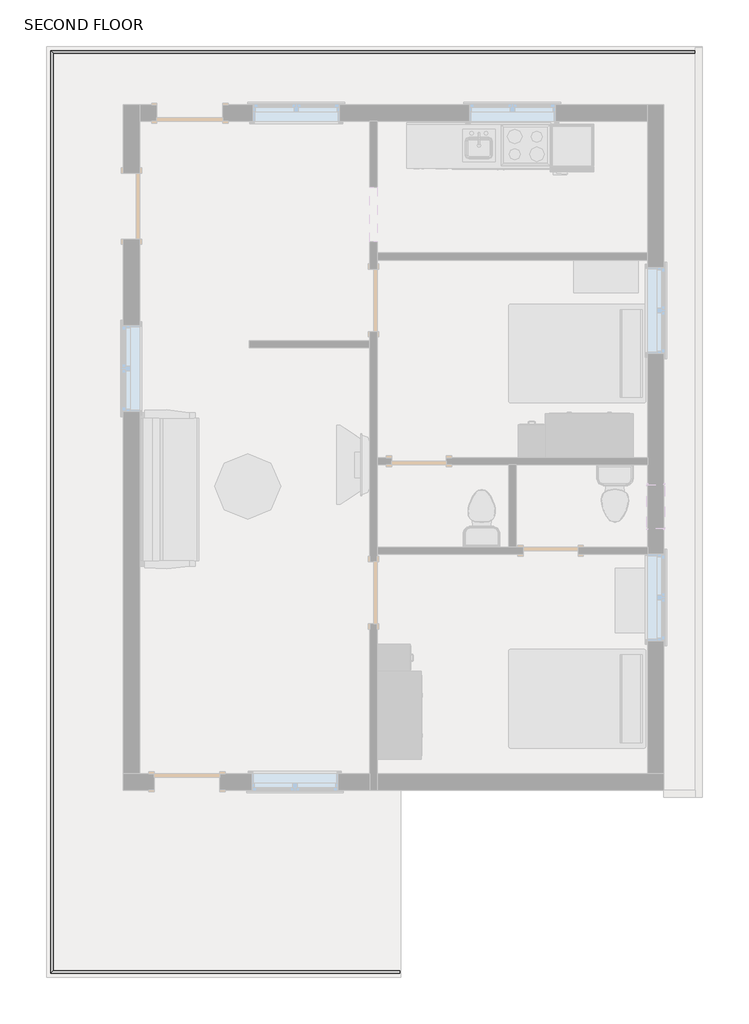
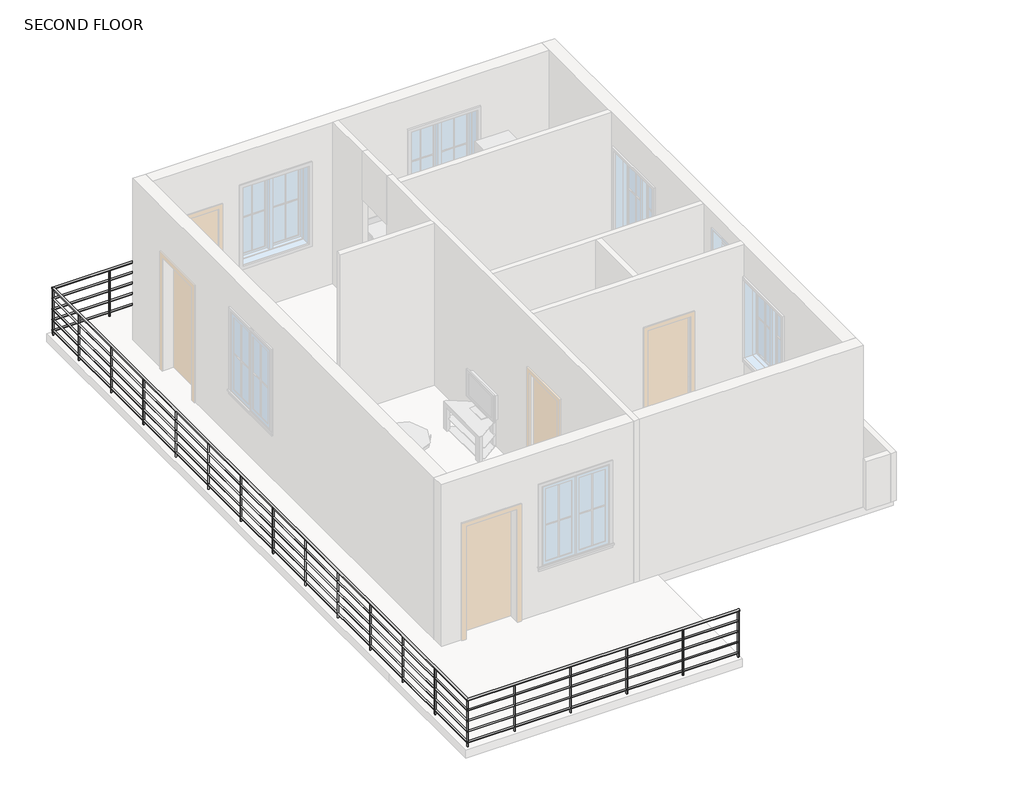
# One storey, part 2 of 3: 1 railing.
"""IFC4 building model written with IfcOpenShell, lengths in millimetres."""

from ifc_helpers import new_model, si_unit, point, frame, frame_2d, origin, place, context, project, spatial, circle_curve, ellipse_curve, trimmed, segment, composite_curve, outline, extrude, element, save
from ifc_brep_helpers import plane_surface, cylinder_surface, advanced_brep

model = new_model("IFC4")

# Units and contexts
model_context = context("Model", 3, world=origin())
ifc_project = project(units=[si_unit("LENGTHUNIT", "METRE", prefix="MILLI")], contexts=[model_context])

# Site, building, storey
site = spatial("IfcSite", under=ifc_project)
building = spatial("IfcBuilding", under=site)
storey = spatial("IfcBuildingStorey", under=building, Name="SECOND FLOOR", Elevation=6400.8)

# Railing
placement = place(None, origin())
element("IfcRailing", 1, ObjectType="900mm Pipe", at=placement, inside=storey, context=model_context, shape_type="SolidModel", body=[
    advanced_brep(
    [(200.9145071, -6925.6741001, 7280.8), (200.9145071, -6965.6741001, 7280.8), (-4655.4544048, -6965.6741001, 7280.8), (-4615.4544048, -6925.6741001, 7280.8), (-4655.4544048, 5865.7351347, 7280.8), (-4615.4544048, 5825.7351347, 7280.8), (4406.9455952, 5825.7351347, 7280.8), (4406.9455952, 5865.7351347, 7280.8)],
    [
        (0, 1, circle_curve(frame((200.9145071, -6945.6741001, 7280.8), z_axis=(1.0, 0.0, 0.0), x_axis=(0.0, -1.0, 0.0)), 20.0)),
        (1, 0, circle_curve(frame((200.9145071, -6945.6741001, 7280.8), z_axis=(1.0, 0.0, 0.0), x_axis=(0.0, -1.0, 0.0)), 20.0)),
        (1, 2),
        (2, 3, ellipse_curve(frame((-4635.4544048, -6945.6741001, 7280.8), z_axis=(0.7071067811865458, -0.7071067811865492, 0.0), x_axis=(0.7071067811865492, 0.7071067811865458, 0.0)), 28.2842712, 20.0)),
        (3, 0),
        (3, 2, ellipse_curve(frame((-4635.4544048, -6945.6741001, 7280.8), z_axis=(0.7071067811865458, -0.7071067811865492, 0.0), x_axis=(0.7071067811865492, 0.7071067811865458, 0.0)), 28.2842712, 20.0)),
        (2, 4),
        (4, 5, ellipse_curve(frame((-4635.4544048, 5845.7351347, 7280.8), z_axis=(-0.7071067811865491, -0.7071067811865459, 0.0), x_axis=(0.7071067811865458, -0.7071067811865491, 0.0)), 28.2842712, 20.0)),
        (5, 3),
        (5, 4, ellipse_curve(frame((-4635.4544048, 5845.7351347, 7280.8), z_axis=(-0.7071067811865491, -0.7071067811865459, 0.0), x_axis=(0.7071067811865458, -0.7071067811865491, 0.0)), 28.2842712, 20.0)),
        (6, 7, circle_curve(frame((4406.9455952, 5845.7351347, 7280.8), z_axis=(1.0, 0.0, 0.0), x_axis=(0.0, 1.0, 0.0)), 20.0)),
        (7, 6, circle_curve(frame((4406.9455952, 5845.7351347, 7280.8), z_axis=(1.0, 0.0, 0.0), x_axis=(0.0, 1.0, 0.0)), 20.0)),
        (4, 7),
        (6, 5),
    ],
    [
        plane_surface(frame((200.9145071, -6945.6741001, 7300.8), z_axis=(1.0, 0.0, 0.0), x_axis=(0.0, -1.0, 0.0))),
        cylinder_surface(frame((200.9145071, -6945.6741001, 7280.8), z_axis=(1.0, 0.0, 0.0), x_axis=(0.0, -1.0, 0.0)), 20.0),
        cylinder_surface(frame((-4635.4544048, -6945.6741001, 7280.8), z_axis=(0.0, -1.0, 0.0), x_axis=(-1.0, 0.0, 0.0)), 20.0),
        plane_surface(frame((4406.9455952, 5845.7351347, 7300.8), z_axis=(1.0, 0.0, 0.0), x_axis=(0.0, 1.0, 0.0))),
        cylinder_surface(frame((-4635.4544048, 5845.7351347, 7280.8), z_axis=(-1.0, 0.0, 0.0), x_axis=(0.0, 1.0, 0.0)), 20.0),
    ],
    [
        (0, [[1, 2]]),
        (1, [[-2, 3, 4, 5]]),
        (1, [[-1, -5, 6, -3]]),
        (2, [[-4, 7, 8, 9]]),
        (2, [[-6, -9, 10, -7]]),
        (3, [[11, 12]]),
        (4, [[-8, 13, -11, 14]]),
        (4, [[-10, -14, -12, -13]]),
    ],
),
    advanced_brep(
    [(200.9145071, -6960.6741001, 7085.8), (200.9145071, -6930.6741001, 7085.8), (4406.9455952, 5860.7351347, 7085.8), (4406.9455952, 5830.7351347, 7085.8), (-4650.4544048, -6960.6741001, 7085.8), (-4620.4544048, -6930.6741001, 7085.8), (-4650.4544048, 5860.7351347, 7085.8), (-4620.4544048, 5830.7351347, 7085.8)],
    [
        (0, 1, circle_curve(frame((200.9145071, -6945.6741001, 7085.8), z_axis=(1.0, 0.0, 0.0), x_axis=(0.0, 1.0, 0.0)), 15.0)),
        (1, 0, circle_curve(frame((200.9145071, -6945.6741001, 7085.8), z_axis=(1.0, 0.0, 0.0), x_axis=(0.0, 1.0, 0.0)), 15.0)),
        (2, 3, circle_curve(frame((4406.9455952, 5845.7351347, 7085.8), z_axis=(1.0, 0.0, 0.0), x_axis=(0.0, -1.0, 0.0)), 15.0)),
        (3, 2, circle_curve(frame((4406.9455952, 5845.7351347, 7085.8), z_axis=(1.0, 0.0, 0.0), x_axis=(0.0, -1.0, 0.0)), 15.0)),
        (0, 4),
        (4, 5, ellipse_curve(frame((-4635.4544048, -6945.6741001, 7085.8), z_axis=(0.7071067811865458, -0.7071067811865492, 0.0), x_axis=(0.7071067811865492, 0.7071067811865458, 0.0)), 21.2132034, 15.0)),
        (5, 1),
        (5, 4, ellipse_curve(frame((-4635.4544048, -6945.6741001, 7085.8), z_axis=(0.7071067811865458, -0.7071067811865492, 0.0), x_axis=(0.7071067811865492, 0.7071067811865458, 0.0)), 21.2132034, 15.0)),
        (4, 6),
        (6, 7, ellipse_curve(frame((-4635.4544048, 5845.7351347, 7085.8), z_axis=(-0.7071067811865491, -0.7071067811865459, 0.0), x_axis=(0.7071067811865458, -0.7071067811865491, 0.0)), 21.2132034, 15.0)),
        (7, 5),
        (7, 6, ellipse_curve(frame((-4635.4544048, 5845.7351347, 7085.8), z_axis=(-0.7071067811865491, -0.7071067811865459, 0.0), x_axis=(0.7071067811865458, -0.7071067811865491, 0.0)), 21.2132034, 15.0)),
        (6, 2),
        (3, 7),
    ],
    [
        plane_surface(frame((200.9145071, -6945.6741001, 7100.8), z_axis=(1.0, 0.0, 0.0), x_axis=(0.0, -1.0, 0.0))),
        plane_surface(frame((4406.9455952, 5845.7351347, 7100.8), z_axis=(1.0, 0.0, 0.0), x_axis=(0.0, 1.0, 0.0))),
        cylinder_surface(frame((200.9145071, -6945.6741001, 7085.8), z_axis=(1.0, 0.0, 0.0), x_axis=(0.0, 1.0, 0.0)), 15.0),
        cylinder_surface(frame((-4635.4544048, -6945.6741001, 7085.8), z_axis=(0.0, -1.0, 0.0), x_axis=(1.0, 0.0, 0.0)), 15.0),
        cylinder_surface(frame((-4635.4544048, 5845.7351347, 7085.8), z_axis=(-1.0, 0.0, 0.0), x_axis=(0.0, -1.0, 0.0)), 15.0),
    ],
    [
        (0, [[1, 2]]),
        (1, [[3, 4]]),
        (2, [[-1, 5, 6, 7]]),
        (2, [[-2, -7, 8, -5]]),
        (3, [[-6, 9, 10, 11]]),
        (3, [[-8, -11, 12, -9]]),
        (4, [[-10, 13, -4, 14]]),
        (4, [[-12, -14, -3, -13]]),
    ],
),
    advanced_brep(
    [(200.9145071, -6960.6741001, 6885.8), (200.9145071, -6930.6741001, 6885.8), (4406.9455952, 5860.7351347, 6885.8), (4406.9455952, 5830.7351347, 6885.8), (-4650.4544048, -6960.6741001, 6885.8), (-4620.4544048, -6930.6741001, 6885.8), (-4650.4544048, 5860.7351347, 6885.8), (-4620.4544048, 5830.7351347, 6885.8)],
    [
        (0, 1, circle_curve(frame((200.9145071, -6945.6741001, 6885.8), z_axis=(1.0, 0.0, 0.0), x_axis=(0.0, 1.0, 0.0)), 15.0)),
        (1, 0, circle_curve(frame((200.9145071, -6945.6741001, 6885.8), z_axis=(1.0, 0.0, 0.0), x_axis=(0.0, 1.0, 0.0)), 15.0)),
        (2, 3, circle_curve(frame((4406.9455952, 5845.7351347, 6885.8), z_axis=(1.0, 0.0, 0.0), x_axis=(0.0, -1.0, 0.0)), 15.0)),
        (3, 2, circle_curve(frame((4406.9455952, 5845.7351347, 6885.8), z_axis=(1.0, 0.0, 0.0), x_axis=(0.0, -1.0, 0.0)), 15.0)),
        (0, 4),
        (4, 5, ellipse_curve(frame((-4635.4544048, -6945.6741001, 6885.8), z_axis=(0.7071067811865458, -0.7071067811865492, 0.0), x_axis=(0.7071067811865492, 0.7071067811865458, 0.0)), 21.2132034, 15.0)),
        (5, 1),
        (5, 4, ellipse_curve(frame((-4635.4544048, -6945.6741001, 6885.8), z_axis=(0.7071067811865458, -0.7071067811865492, 0.0), x_axis=(0.7071067811865492, 0.7071067811865458, 0.0)), 21.2132034, 15.0)),
        (4, 6),
        (6, 7, ellipse_curve(frame((-4635.4544048, 5845.7351347, 6885.8), z_axis=(-0.7071067811865491, -0.7071067811865459, 0.0), x_axis=(0.7071067811865458, -0.7071067811865491, 0.0)), 21.2132034, 15.0)),
        (7, 5),
        (7, 6, ellipse_curve(frame((-4635.4544048, 5845.7351347, 6885.8), z_axis=(-0.7071067811865491, -0.7071067811865459, 0.0), x_axis=(0.7071067811865458, -0.7071067811865491, 0.0)), 21.2132034, 15.0)),
        (6, 2),
        (3, 7),
    ],
    [
        plane_surface(frame((200.9145071, -6945.6741001, 6900.8), z_axis=(1.0, 0.0, 0.0), x_axis=(0.0, -1.0, 0.0))),
        plane_surface(frame((4406.9455952, 5845.7351347, 6900.8), z_axis=(1.0, 0.0, 0.0), x_axis=(0.0, 1.0, 0.0))),
        cylinder_surface(frame((200.9145071, -6945.6741001, 6885.8), z_axis=(1.0, 0.0, 0.0), x_axis=(0.0, 1.0, 0.0)), 15.0),
        cylinder_surface(frame((-4635.4544048, -6945.6741001, 6885.8), z_axis=(0.0, -1.0, 0.0), x_axis=(1.0, 0.0, 0.0)), 15.0),
        cylinder_surface(frame((-4635.4544048, 5845.7351347, 6885.8), z_axis=(-1.0, 0.0, 0.0), x_axis=(0.0, -1.0, 0.0)), 15.0),
    ],
    [
        (0, [[1, 2]]),
        (1, [[3, 4]]),
        (2, [[-1, 5, 6, 7]]),
        (2, [[-2, -7, 8, -5]]),
        (3, [[-6, 9, 10, 11]]),
        (3, [[-8, -11, 12, -9]]),
        (4, [[-10, 13, -4, 14]]),
        (4, [[-12, -14, -3, -13]]),
    ],
),
    advanced_brep(
    [(200.9145071, -6960.6741001, 6685.8), (200.9145071, -6930.6741001, 6685.8), (-4650.4544048, -6960.6741001, 6685.8), (-4620.4544048, -6930.6741001, 6685.8), (-4650.4544048, 5860.7351347, 6685.8), (-4620.4544048, 5830.7351347, 6685.8), (4406.9455952, 5860.7351347, 6685.8), (4406.9455952, 5830.7351347, 6685.8)],
    [
        (0, 1, circle_curve(frame((200.9145071, -6945.6741001, 6685.8), z_axis=(1.0, 0.0, 0.0), x_axis=(0.0, 1.0, 0.0)), 15.0)),
        (1, 0, circle_curve(frame((200.9145071, -6945.6741001, 6685.8), z_axis=(1.0, 0.0, 0.0), x_axis=(0.0, 1.0, 0.0)), 15.0)),
        (0, 2),
        (2, 3, ellipse_curve(frame((-4635.4544048, -6945.6741001, 6685.8), z_axis=(0.7071067811865458, -0.7071067811865492, 0.0), x_axis=(0.7071067811865492, 0.7071067811865458, 0.0)), 21.2132034, 15.0)),
        (3, 1),
        (3, 2, ellipse_curve(frame((-4635.4544048, -6945.6741001, 6685.8), z_axis=(0.7071067811865458, -0.7071067811865492, 0.0), x_axis=(0.7071067811865492, 0.7071067811865458, 0.0)), 21.2132034, 15.0)),
        (2, 4),
        (4, 5, ellipse_curve(frame((-4635.4544048, 5845.7351347, 6685.8), z_axis=(-0.7071067811865491, -0.7071067811865459, 0.0), x_axis=(0.7071067811865458, -0.7071067811865491, 0.0)), 21.2132034, 15.0)),
        (5, 3),
        (5, 4, ellipse_curve(frame((-4635.4544048, 5845.7351347, 6685.8), z_axis=(-0.7071067811865491, -0.7071067811865459, 0.0), x_axis=(0.7071067811865458, -0.7071067811865491, 0.0)), 21.2132034, 15.0)),
        (6, 7, circle_curve(frame((4406.9455952, 5845.7351347, 6685.8), z_axis=(1.0, 0.0, 0.0), x_axis=(0.0, -1.0, 0.0)), 15.0)),
        (7, 6, circle_curve(frame((4406.9455952, 5845.7351347, 6685.8), z_axis=(1.0, 0.0, 0.0), x_axis=(0.0, -1.0, 0.0)), 15.0)),
        (4, 6),
        (7, 5),
    ],
    [
        plane_surface(frame((200.9145071, -6945.6741001, 6700.8), z_axis=(1.0, 0.0, 0.0), x_axis=(0.0, -1.0, 0.0))),
        cylinder_surface(frame((200.9145071, -6945.6741001, 6685.8), z_axis=(1.0, 0.0, 0.0), x_axis=(0.0, 1.0, 0.0)), 15.0),
        cylinder_surface(frame((-4635.4544048, -6945.6741001, 6685.8), z_axis=(0.0, -1.0, 0.0), x_axis=(1.0, 0.0, 0.0)), 15.0),
        plane_surface(frame((4406.9455952, 5845.7351347, 6700.8), z_axis=(1.0, 0.0, 0.0), x_axis=(0.0, 1.0, 0.0))),
        cylinder_surface(frame((-4635.4544048, 5845.7351347, 6685.8), z_axis=(-1.0, 0.0, 0.0), x_axis=(0.0, -1.0, 0.0)), 15.0),
    ],
    [
        (0, [[1, 2]]),
        (1, [[-1, 3, 4, 5]]),
        (1, [[-2, -5, 6, -3]]),
        (2, [[-4, 7, 8, 9]]),
        (2, [[-6, -9, 10, -7]]),
        (3, [[11, 12]]),
        (4, [[-8, 13, -12, 14]]),
        (4, [[-10, -14, -11, -13]]),
    ],
),
    advanced_brep(
    [(200.9145071, -6960.6741001, 6485.8), (200.9145071, -6930.6741001, 6485.8), (-4650.4544048, -6960.6741001, 6485.8), (-4620.4544048, -6930.6741001, 6485.8), (-4650.4544048, 5860.7351347, 6485.8), (-4620.4544048, 5830.7351347, 6485.8), (4406.9455952, 5860.7351347, 6485.8), (4406.9455952, 5830.7351347, 6485.8)],
    [
        (0, 1, circle_curve(frame((200.9145071, -6945.6741001, 6485.8), z_axis=(1.0, 0.0, 0.0), x_axis=(0.0, 1.0, 0.0)), 15.0)),
        (1, 0, circle_curve(frame((200.9145071, -6945.6741001, 6485.8), z_axis=(1.0, 0.0, 0.0), x_axis=(0.0, 1.0, 0.0)), 15.0)),
        (0, 2),
        (2, 3, ellipse_curve(frame((-4635.4544048, -6945.6741001, 6485.8), z_axis=(0.7071067811865458, -0.7071067811865492, 0.0), x_axis=(0.7071067811865492, 0.7071067811865458, 0.0)), 21.2132034, 15.0)),
        (3, 1),
        (3, 2, ellipse_curve(frame((-4635.4544048, -6945.6741001, 6485.8), z_axis=(0.7071067811865458, -0.7071067811865492, 0.0), x_axis=(0.7071067811865492, 0.7071067811865458, 0.0)), 21.2132034, 15.0)),
        (2, 4),
        (4, 5, ellipse_curve(frame((-4635.4544048, 5845.7351347, 6485.8), z_axis=(-0.7071067811865491, -0.7071067811865459, 0.0), x_axis=(0.7071067811865458, -0.7071067811865491, 0.0)), 21.2132034, 15.0)),
        (5, 3),
        (5, 4, ellipse_curve(frame((-4635.4544048, 5845.7351347, 6485.8), z_axis=(-0.7071067811865491, -0.7071067811865459, 0.0), x_axis=(0.7071067811865458, -0.7071067811865491, 0.0)), 21.2132034, 15.0)),
        (6, 7, circle_curve(frame((4406.9455952, 5845.7351347, 6485.8), z_axis=(1.0, 0.0, 0.0), x_axis=(0.0, -1.0, 0.0)), 15.0)),
        (7, 6, circle_curve(frame((4406.9455952, 5845.7351347, 6485.8), z_axis=(1.0, 0.0, 0.0), x_axis=(0.0, -1.0, 0.0)), 15.0)),
        (4, 6),
        (7, 5),
    ],
    [
        plane_surface(frame((200.9145071, -6945.6741001, 6500.8), z_axis=(1.0, 0.0, 0.0), x_axis=(0.0, -1.0, 0.0))),
        cylinder_surface(frame((200.9145071, -6945.6741001, 6485.8), z_axis=(1.0, 0.0, 0.0), x_axis=(0.0, 1.0, 0.0)), 15.0),
        cylinder_surface(frame((-4635.4544048, -6945.6741001, 6485.8), z_axis=(0.0, -1.0, 0.0), x_axis=(1.0, 0.0, 0.0)), 15.0),
        plane_surface(frame((4406.9455952, 5845.7351347, 6500.8), z_axis=(1.0, 0.0, 0.0), x_axis=(0.0, 1.0, 0.0))),
        cylinder_surface(frame((-4635.4544048, 5845.7351347, 6485.8), z_axis=(-1.0, 0.0, 0.0), x_axis=(0.0, -1.0, 0.0)), 15.0),
    ],
    [
        (0, [[1, 2]]),
        (1, [[-1, 3, 4, 5]]),
        (1, [[-2, -5, 6, -3]]),
        (2, [[-4, 7, 8, 9]]),
        (2, [[-6, -9, 10, -7]]),
        (3, [[11, 12]]),
        (4, [[-8, 13, -12, 14]]),
        (4, [[-10, -14, -11, -13]]),
    ],
),
    extrude(outline(composite_curve([segment(trimmed(circle_curve(frame_2d((4364.5455952, 5845.7351347)), 12.5), [point((4364.5455952, 5858.2351347))], [point((4364.5455952, 5833.2351347))], False, "CARTESIAN"), True, "CONTINUOUS"), segment(trimmed(circle_curve(frame_2d((4364.5455952, 5845.7351347)), 12.5), [point((4364.5455952, 5833.2351347))], [point((4364.5455952, 5858.2351347))], False, "CARTESIAN"), True, "CONTINUOUS")], self_intersect=False)), frame((0.0, 0.0, 6400.8), z_axis=(0.0, 0.0, 1.0), x_axis=(1.0, 0.0, 0.0)), (0.0, 0.0, 1.0), 860.0),
    extrude(outline(composite_curve([segment(trimmed(circle_curve(frame_2d((3364.5455952, 5845.7351347)), 12.5), [point((3364.5455952, 5858.2351347))], [point((3364.5455952, 5833.2351347))], False, "CARTESIAN"), True, "CONTINUOUS"), segment(trimmed(circle_curve(frame_2d((3364.5455952, 5845.7351347)), 12.5), [point((3364.5455952, 5833.2351347))], [point((3364.5455952, 5858.2351347))], False, "CARTESIAN"), True, "CONTINUOUS")], self_intersect=False)), frame((0.0, 0.0, 6400.8), z_axis=(0.0, 0.0, 1.0), x_axis=(1.0, 0.0, 0.0)), (0.0, 0.0, 1.0), 860.0),
    extrude(outline(composite_curve([segment(trimmed(circle_curve(frame_2d((2364.5455952, 5845.7351347)), 12.5), [point((2364.5455952, 5858.2351347))], [point((2364.5455952, 5833.2351347))], False, "CARTESIAN"), True, "CONTINUOUS"), segment(trimmed(circle_curve(frame_2d((2364.5455952, 5845.7351347)), 12.5), [point((2364.5455952, 5833.2351347))], [point((2364.5455952, 5858.2351347))], False, "CARTESIAN"), True, "CONTINUOUS")], self_intersect=False)), frame((0.0, 0.0, 6400.8), z_axis=(0.0, 0.0, 1.0), x_axis=(1.0, 0.0, 0.0)), (0.0, 0.0, 1.0), 860.0),
    extrude(outline(composite_curve([segment(trimmed(circle_curve(frame_2d((1364.5455952, 5845.7351347)), 12.5), [point((1364.5455952, 5858.2351347))], [point((1364.5455952, 5833.2351347))], False, "CARTESIAN"), True, "CONTINUOUS"), segment(trimmed(circle_curve(frame_2d((1364.5455952, 5845.7351347)), 12.5), [point((1364.5455952, 5833.2351347))], [point((1364.5455952, 5858.2351347))], False, "CARTESIAN"), True, "CONTINUOUS")], self_intersect=False)), frame((0.0, 0.0, 6400.8), z_axis=(0.0, 0.0, 1.0), x_axis=(1.0, 0.0, 0.0)), (0.0, 0.0, 1.0), 860.0),
    extrude(outline(composite_curve([segment(trimmed(circle_curve(frame_2d((364.5455952, 5845.7351347)), 12.5), [point((364.5455952, 5858.2351347))], [point((364.5455952, 5833.2351347))], False, "CARTESIAN"), True, "CONTINUOUS"), segment(trimmed(circle_curve(frame_2d((364.5455952, 5845.7351347)), 12.5), [point((364.5455952, 5833.2351347))], [point((364.5455952, 5858.2351347))], False, "CARTESIAN"), True, "CONTINUOUS")], self_intersect=False)), frame((0.0, 0.0, 6400.8), z_axis=(0.0, 0.0, 1.0), x_axis=(1.0, 0.0, 0.0)), (0.0, 0.0, 1.0), 860.0),
    extrude(outline(composite_curve([segment(trimmed(circle_curve(frame_2d((-635.4544048, 5845.7351347)), 12.5), [point((-635.4544048, 5858.2351347))], [point((-635.4544048, 5833.2351347))], False, "CARTESIAN"), True, "CONTINUOUS"), segment(trimmed(circle_curve(frame_2d((-635.4544048, 5845.7351347)), 12.5), [point((-635.4544048, 5833.2351347))], [point((-635.4544048, 5858.2351347))], False, "CARTESIAN"), True, "CONTINUOUS")], self_intersect=False)), frame((0.0, 0.0, 6400.8), z_axis=(0.0, 0.0, 1.0), x_axis=(1.0, 0.0, 0.0)), (0.0, 0.0, 1.0), 860.0),
    extrude(outline(composite_curve([segment(trimmed(circle_curve(frame_2d((-1635.4544048, 5845.7351347)), 12.5), [point((-1635.4544048, 5858.2351347))], [point((-1635.4544048, 5833.2351347))], False, "CARTESIAN"), True, "CONTINUOUS"), segment(trimmed(circle_curve(frame_2d((-1635.4544048, 5845.7351347)), 12.5), [point((-1635.4544048, 5833.2351347))], [point((-1635.4544048, 5858.2351347))], False, "CARTESIAN"), True, "CONTINUOUS")], self_intersect=False)), frame((0.0, 0.0, 6400.8), z_axis=(0.0, 0.0, 1.0), x_axis=(1.0, 0.0, 0.0)), (0.0, 0.0, 1.0), 860.0),
    extrude(outline(composite_curve([segment(trimmed(circle_curve(frame_2d((-2635.4544048, 5845.7351347)), 12.5), [point((-2635.4544048, 5858.2351347))], [point((-2635.4544048, 5833.2351347))], False, "CARTESIAN"), True, "CONTINUOUS"), segment(trimmed(circle_curve(frame_2d((-2635.4544048, 5845.7351347)), 12.5), [point((-2635.4544048, 5833.2351347))], [point((-2635.4544048, 5858.2351347))], False, "CARTESIAN"), True, "CONTINUOUS")], self_intersect=False)), frame((0.0, 0.0, 6400.8), z_axis=(0.0, 0.0, 1.0), x_axis=(1.0, 0.0, 0.0)), (0.0, 0.0, 1.0), 860.0),
    extrude(outline(composite_curve([segment(trimmed(circle_curve(frame_2d((-3635.4544048, 5845.7351347)), 12.5), [point((-3635.4544048, 5858.2351347))], [point((-3635.4544048, 5833.2351347))], False, "CARTESIAN"), True, "CONTINUOUS"), segment(trimmed(circle_curve(frame_2d((-3635.4544048, 5845.7351347)), 12.5), [point((-3635.4544048, 5833.2351347))], [point((-3635.4544048, 5858.2351347))], False, "CARTESIAN"), True, "CONTINUOUS")], self_intersect=False)), frame((0.0, 0.0, 6400.8), z_axis=(0.0, 0.0, 1.0), x_axis=(1.0, 0.0, 0.0)), (0.0, 0.0, 1.0), 860.0),
    extrude(outline(composite_curve([segment(trimmed(circle_curve(frame_2d((-4635.4544048, 5054.3258999)), 12.5), [point((-4647.9544048, 5054.3258999))], [point((-4622.9544048, 5054.3258999))], False, "CARTESIAN"), True, "CONTINUOUS"), segment(trimmed(circle_curve(frame_2d((-4635.4544048, 5054.3258999)), 12.5), [point((-4622.9544048, 5054.3258999))], [point((-4647.9544048, 5054.3258999))], False, "CARTESIAN"), True, "CONTINUOUS")], self_intersect=False)), frame((0.0, 0.0, 6400.8), z_axis=(0.0, 0.0, 1.0), x_axis=(1.0, 0.0, 0.0)), (0.0, 0.0, 1.0), 860.0),
    extrude(outline(composite_curve([segment(trimmed(circle_curve(frame_2d((-4635.4544048, 4054.3258999)), 12.5), [point((-4647.9544048, 4054.3258999))], [point((-4622.9544048, 4054.3258999))], False, "CARTESIAN"), True, "CONTINUOUS"), segment(trimmed(circle_curve(frame_2d((-4635.4544048, 4054.3258999)), 12.5), [point((-4622.9544048, 4054.3258999))], [point((-4647.9544048, 4054.3258999))], False, "CARTESIAN"), True, "CONTINUOUS")], self_intersect=False)), frame((0.0, 0.0, 6400.8), z_axis=(0.0, 0.0, 1.0), x_axis=(1.0, 0.0, 0.0)), (0.0, 0.0, 1.0), 860.0),
    extrude(outline(composite_curve([segment(trimmed(circle_curve(frame_2d((-4635.4544048, 3054.3258999)), 12.5), [point((-4647.9544048, 3054.3258999))], [point((-4622.9544048, 3054.3258999))], False, "CARTESIAN"), True, "CONTINUOUS"), segment(trimmed(circle_curve(frame_2d((-4635.4544048, 3054.3258999)), 12.5), [point((-4622.9544048, 3054.3258999))], [point((-4647.9544048, 3054.3258999))], False, "CARTESIAN"), True, "CONTINUOUS")], self_intersect=False)), frame((0.0, 0.0, 6400.8), z_axis=(0.0, 0.0, 1.0), x_axis=(1.0, 0.0, 0.0)), (0.0, 0.0, 1.0), 860.0),
    extrude(outline(composite_curve([segment(trimmed(circle_curve(frame_2d((-4635.4544048, 2054.3258999)), 12.5), [point((-4647.9544048, 2054.3258999))], [point((-4622.9544048, 2054.3258999))], False, "CARTESIAN"), True, "CONTINUOUS"), segment(trimmed(circle_curve(frame_2d((-4635.4544048, 2054.3258999)), 12.5), [point((-4622.9544048, 2054.3258999))], [point((-4647.9544048, 2054.3258999))], False, "CARTESIAN"), True, "CONTINUOUS")], self_intersect=False)), frame((0.0, 0.0, 6400.8), z_axis=(0.0, 0.0, 1.0), x_axis=(1.0, 0.0, 0.0)), (0.0, 0.0, 1.0), 860.0),
    extrude(outline(composite_curve([segment(trimmed(circle_curve(frame_2d((-4635.4544048, 1054.3258999)), 12.5), [point((-4647.9544048, 1054.3258999))], [point((-4622.9544048, 1054.3258999))], False, "CARTESIAN"), True, "CONTINUOUS"), segment(trimmed(circle_curve(frame_2d((-4635.4544048, 1054.3258999)), 12.5), [point((-4622.9544048, 1054.3258999))], [point((-4647.9544048, 1054.3258999))], False, "CARTESIAN"), True, "CONTINUOUS")], self_intersect=False)), frame((0.0, 0.0, 6400.8), z_axis=(0.0, 0.0, 1.0), x_axis=(1.0, 0.0, 0.0)), (0.0, 0.0, 1.0), 860.0),
    extrude(outline(composite_curve([segment(trimmed(circle_curve(frame_2d((-4635.4544048, 54.3258999)), 12.5), [point((-4647.9544048, 54.3258999))], [point((-4622.9544048, 54.3258999))], False, "CARTESIAN"), True, "CONTINUOUS"), segment(trimmed(circle_curve(frame_2d((-4635.4544048, 54.3258999)), 12.5), [point((-4622.9544048, 54.3258999))], [point((-4647.9544048, 54.3258999))], False, "CARTESIAN"), True, "CONTINUOUS")], self_intersect=False)), frame((0.0, 0.0, 6400.8), z_axis=(0.0, 0.0, 1.0), x_axis=(1.0, 0.0, 0.0)), (0.0, 0.0, 1.0), 860.0),
    extrude(outline(composite_curve([segment(trimmed(circle_curve(frame_2d((-4635.4544048, -945.6741001)), 12.5), [point((-4647.9544048, -945.6741001))], [point((-4622.9544048, -945.6741001))], False, "CARTESIAN"), True, "CONTINUOUS"), segment(trimmed(circle_curve(frame_2d((-4635.4544048, -945.6741001)), 12.5), [point((-4622.9544048, -945.6741001))], [point((-4647.9544048, -945.6741001))], False, "CARTESIAN"), True, "CONTINUOUS")], self_intersect=False)), frame((0.0, 0.0, 6400.8), z_axis=(0.0, 0.0, 1.0), x_axis=(1.0, 0.0, 0.0)), (0.0, 0.0, 1.0), 860.0),
    extrude(outline(composite_curve([segment(trimmed(circle_curve(frame_2d((-4635.4544048, -1945.6741001)), 12.5), [point((-4647.9544048, -1945.6741001))], [point((-4622.9544048, -1945.6741001))], False, "CARTESIAN"), True, "CONTINUOUS"), segment(trimmed(circle_curve(frame_2d((-4635.4544048, -1945.6741001)), 12.5), [point((-4622.9544048, -1945.6741001))], [point((-4647.9544048, -1945.6741001))], False, "CARTESIAN"), True, "CONTINUOUS")], self_intersect=False)), frame((0.0, 0.0, 6400.8), z_axis=(0.0, 0.0, 1.0), x_axis=(1.0, 0.0, 0.0)), (0.0, 0.0, 1.0), 860.0),
    extrude(outline(composite_curve([segment(trimmed(circle_curve(frame_2d((-4635.4544048, -2945.6741001)), 12.5), [point((-4647.9544048, -2945.6741001))], [point((-4622.9544048, -2945.6741001))], False, "CARTESIAN"), True, "CONTINUOUS"), segment(trimmed(circle_curve(frame_2d((-4635.4544048, -2945.6741001)), 12.5), [point((-4622.9544048, -2945.6741001))], [point((-4647.9544048, -2945.6741001))], False, "CARTESIAN"), True, "CONTINUOUS")], self_intersect=False)), frame((0.0, 0.0, 6400.8), z_axis=(0.0, 0.0, 1.0), x_axis=(1.0, 0.0, 0.0)), (0.0, 0.0, 1.0), 860.0),
    extrude(outline(composite_curve([segment(trimmed(circle_curve(frame_2d((-4635.4544048, -3945.6741001)), 12.5), [point((-4647.9544048, -3945.6741001))], [point((-4622.9544048, -3945.6741001))], False, "CARTESIAN"), True, "CONTINUOUS"), segment(trimmed(circle_curve(frame_2d((-4635.4544048, -3945.6741001)), 12.5), [point((-4622.9544048, -3945.6741001))], [point((-4647.9544048, -3945.6741001))], False, "CARTESIAN"), True, "CONTINUOUS")], self_intersect=False)), frame((0.0, 0.0, 6400.8), z_axis=(0.0, 0.0, 1.0), x_axis=(1.0, 0.0, 0.0)), (0.0, 0.0, 1.0), 860.0),
    extrude(outline(composite_curve([segment(trimmed(circle_curve(frame_2d((-4635.4544048, -4945.6741001)), 12.5), [point((-4647.9544048, -4945.6741001))], [point((-4622.9544048, -4945.6741001))], False, "CARTESIAN"), True, "CONTINUOUS"), segment(trimmed(circle_curve(frame_2d((-4635.4544048, -4945.6741001)), 12.5), [point((-4622.9544048, -4945.6741001))], [point((-4647.9544048, -4945.6741001))], False, "CARTESIAN"), True, "CONTINUOUS")], self_intersect=False)), frame((0.0, 0.0, 6400.8), z_axis=(0.0, 0.0, 1.0), x_axis=(1.0, 0.0, 0.0)), (0.0, 0.0, 1.0), 860.0),
    extrude(outline(composite_curve([segment(trimmed(circle_curve(frame_2d((-4635.4544048, -5945.6741001)), 12.5), [point((-4647.9544048, -5945.6741001))], [point((-4622.9544048, -5945.6741001))], False, "CARTESIAN"), True, "CONTINUOUS"), segment(trimmed(circle_curve(frame_2d((-4635.4544048, -5945.6741001)), 12.5), [point((-4622.9544048, -5945.6741001))], [point((-4647.9544048, -5945.6741001))], False, "CARTESIAN"), True, "CONTINUOUS")], self_intersect=False)), frame((0.0, 0.0, 6400.8), z_axis=(0.0, 0.0, 1.0), x_axis=(1.0, 0.0, 0.0)), (0.0, 0.0, 1.0), 860.0),
    extrude(outline(composite_curve([segment(trimmed(circle_curve(frame_2d((-3799.0854929, -6945.6741001)), 12.5), [point((-3799.0854929, -6958.1741001))], [point((-3799.0854929, -6933.1741001))], False, "CARTESIAN"), True, "CONTINUOUS"), segment(trimmed(circle_curve(frame_2d((-3799.0854929, -6945.6741001)), 12.5), [point((-3799.0854929, -6933.1741001))], [point((-3799.0854929, -6958.1741001))], False, "CARTESIAN"), True, "CONTINUOUS")], self_intersect=False)), frame((0.0, 0.0, 6400.8), z_axis=(0.0, 0.0, 1.0), x_axis=(1.0, 0.0, 0.0)), (0.0, 0.0, 1.0), 860.0),
    extrude(outline(composite_curve([segment(trimmed(circle_curve(frame_2d((-2799.0854929, -6945.6741001)), 12.5), [point((-2799.0854929, -6958.1741001))], [point((-2799.0854929, -6933.1741001))], False, "CARTESIAN"), True, "CONTINUOUS"), segment(trimmed(circle_curve(frame_2d((-2799.0854929, -6945.6741001)), 12.5), [point((-2799.0854929, -6933.1741001))], [point((-2799.0854929, -6958.1741001))], False, "CARTESIAN"), True, "CONTINUOUS")], self_intersect=False)), frame((0.0, 0.0, 6400.8), z_axis=(0.0, 0.0, 1.0), x_axis=(1.0, 0.0, 0.0)), (0.0, 0.0, 1.0), 860.0),
    extrude(outline(composite_curve([segment(trimmed(circle_curve(frame_2d((-1799.0854929, -6945.6741001)), 12.5), [point((-1799.0854929, -6958.1741001))], [point((-1799.0854929, -6933.1741001))], False, "CARTESIAN"), True, "CONTINUOUS"), segment(trimmed(circle_curve(frame_2d((-1799.0854929, -6945.6741001)), 12.5), [point((-1799.0854929, -6933.1741001))], [point((-1799.0854929, -6958.1741001))], False, "CARTESIAN"), True, "CONTINUOUS")], self_intersect=False)), frame((0.0, 0.0, 6400.8), z_axis=(0.0, 0.0, 1.0), x_axis=(1.0, 0.0, 0.0)), (0.0, 0.0, 1.0), 860.0),
    extrude(outline(composite_curve([segment(trimmed(circle_curve(frame_2d((-799.0854929, -6945.6741001)), 12.5), [point((-799.0854929, -6958.1741001))], [point((-799.0854929, -6933.1741001))], False, "CARTESIAN"), True, "CONTINUOUS"), segment(trimmed(circle_curve(frame_2d((-799.0854929, -6945.6741001)), 12.5), [point((-799.0854929, -6933.1741001))], [point((-799.0854929, -6958.1741001))], False, "CARTESIAN"), True, "CONTINUOUS")], self_intersect=False)), frame((0.0, 0.0, 6400.8), z_axis=(0.0, 0.0, 1.0), x_axis=(1.0, 0.0, 0.0)), (0.0, 0.0, 1.0), 860.0),
    extrude(outline(composite_curve([segment(trimmed(circle_curve(frame_2d((-4635.4544048, 5845.7351347)), 12.5), [point((-4647.9544048, 5845.7351347))], [point((-4622.9544048, 5845.7351347))], False, "CARTESIAN"), True, "CONTINUOUS"), segment(trimmed(circle_curve(frame_2d((-4635.4544048, 5845.7351347)), 12.5), [point((-4622.9544048, 5845.7351347))], [point((-4647.9544048, 5845.7351347))], False, "CARTESIAN"), True, "CONTINUOUS")], self_intersect=False)), frame((0.0, 0.0, 6400.8), z_axis=(0.0, 0.0, 1.0), x_axis=(1.0, 0.0, 0.0)), (0.0, 0.0, 1.0), 860.0),
    extrude(outline(composite_curve([segment(trimmed(circle_curve(frame_2d((-4635.4544048, -6945.6741001)), 12.5), [point((-4635.4544048, -6958.1741001))], [point((-4635.4544048, -6933.1741001))], False, "CARTESIAN"), True, "CONTINUOUS"), segment(trimmed(circle_curve(frame_2d((-4635.4544048, -6945.6741001)), 12.5), [point((-4635.4544048, -6933.1741001))], [point((-4635.4544048, -6958.1741001))], False, "CARTESIAN"), True, "CONTINUOUS")], self_intersect=False)), frame((0.0, 0.0, 6400.8), z_axis=(0.0, 0.0, 1.0), x_axis=(1.0, 0.0, 0.0)), (0.0, 0.0, 1.0), 860.0),
    extrude(outline(composite_curve([segment(trimmed(circle_curve(frame_2d((4394.4455952, 5845.7351347)), 12.5), [point((4394.4455952, 5858.2351347))], [point((4394.4455952, 5833.2351347))], False, "CARTESIAN"), True, "CONTINUOUS"), segment(trimmed(circle_curve(frame_2d((4394.4455952, 5845.7351347)), 12.5), [point((4394.4455952, 5833.2351347))], [point((4394.4455952, 5858.2351347))], False, "CARTESIAN"), True, "CONTINUOUS")], self_intersect=False)), frame((0.0, 0.0, 6400.8), z_axis=(0.0, 0.0, 1.0), x_axis=(1.0, 0.0, 0.0)), (0.0, 0.0, 1.0), 860.0),
    extrude(outline(composite_curve([segment(trimmed(circle_curve(frame_2d((188.4145071, -6945.6741001)), 12.5), [point((188.4145071, -6958.1741001))], [point((188.4145071, -6933.1741001))], False, "CARTESIAN"), True, "CONTINUOUS"), segment(trimmed(circle_curve(frame_2d((188.4145071, -6945.6741001)), 12.5), [point((188.4145071, -6933.1741001))], [point((188.4145071, -6958.1741001))], False, "CARTESIAN"), True, "CONTINUOUS")], self_intersect=False)), frame((0.0, 0.0, 6400.8), z_axis=(0.0, 0.0, 1.0), x_axis=(1.0, 0.0, 0.0)), (0.0, 0.0, 1.0), 860.0),
])

save(model, "model.ifc")

# Revit data of these elements
# Type "900mm Pipe"
#   built-in parameter 1008612 = 0.019685 (stored number, unit not read)
#   built-in parameter 1008611 = 0.0984252 (stored number, unit not read)
#   built-in parameter 1008609 = 3.28084 (stored number, unit not read)
#   built-in parameter 1008604 = 0.19685 (stored number, unit not read)
#   built-in parameter 1008603 = 0.164042 (stored number, unit not read)
#   Railing Height = 2.952756 ft
#   built-in parameter 1008630 = 2
#   built-in parameter 1008610 = 1
#   built-in parameter 1008605 = 1
#   built-in parameter 1008618 = M_Baluster - Round : 25mm
# Element 1 (IfcRailing, "900mm Pipe")
#   Phase Created = New Construction
